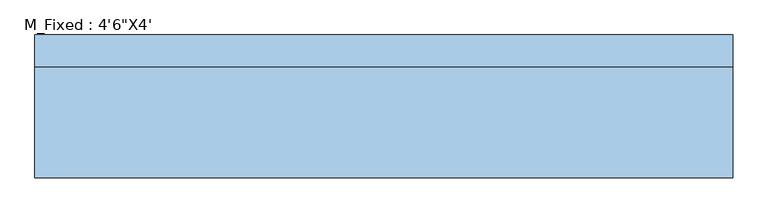
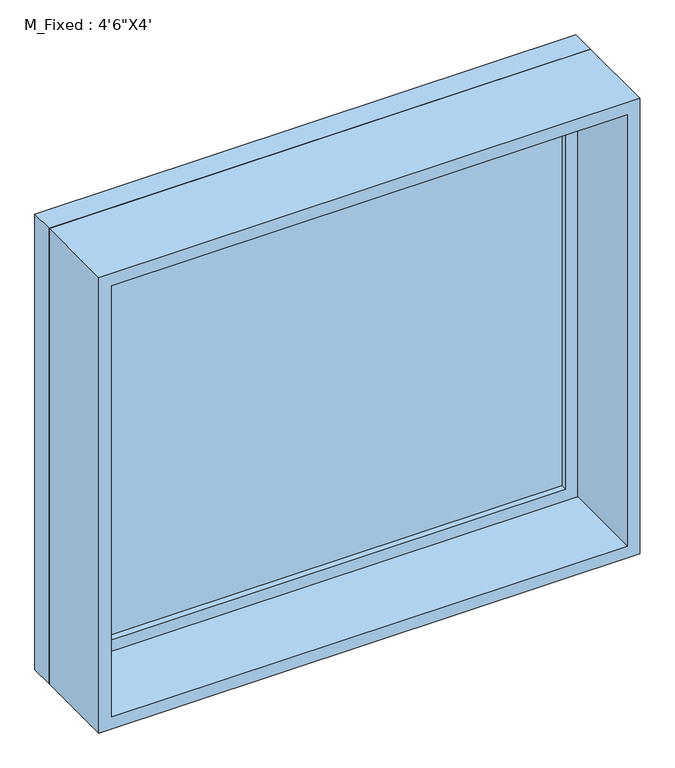
"""IFC4 building model written with IfcOpenShell, lengths in millimetres: window geometry."""

from ifc_helpers import new_model, si_unit, frame, origin, place, context, project, spatial, polyline, outline, extrude, source, transform, mapped, element, save


def window_6cb3df29(model_context):
    return source(origin(), model_context, "Body", "SweptSolid", [
        extrude(outline(polyline([(-622.8, 118.4), (622.8, 118.4), (622.8, 106.4), (-622.8, 106.4), (-622.8, 118.4)])), frame((0.0, 0.0, 977.4), z_axis=(0.0, 0.0, 1.0), x_axis=(1.0, 0.0, 0.0)), (0.0, 0.0, 1.0), 1093.2),
        extrude(outline(polyline([(2114.6, -666.8), (933.4, -666.8), (933.4, 666.8), (2114.6, 666.8), (2114.6, -666.8)]), holes=[polyline([(2070.6, -622.8), (2070.6, 622.8), (977.4, 622.8), (977.4, -622.8), (2070.6, -622.8)])]), frame((0.0, 90.4, 0.0), z_axis=(0.0, 1.0, 0.0), x_axis=(0.0, 0.0, 1.0)), (0.0, 0.0, 1.0), 44.0),
        extrude(outline(polyline([(2133.6, -685.8), (914.4, -685.8), (914.4, 685.8), (2133.6, 685.8), (2133.6, -685.8)]), holes=[polyline([(2114.6, -666.8), (2114.6, 666.8), (933.4, 666.8), (933.4, -666.8), (2114.6, -666.8)])]), frame((0.0, 90.4, 0.0), z_axis=(0.0, 1.0, 0.0), x_axis=(0.0, 0.0, 1.0)), (0.0, 0.0, 1.0), 63.0),
        extrude(outline(polyline([(2133.6, -685.8), (914.4, -685.8), (914.4, 685.8), (2133.6, 685.8), (2133.6, -685.8)]), holes=[polyline([(2101.6, -653.8), (2101.6, 653.8), (946.4, 653.8), (946.4, -653.8), (2101.6, -653.8)])]), frame((0.0, -127.4, 0.0), z_axis=(0.0, 1.0, 0.0), x_axis=(0.0, 0.0, 1.0)), (0.0, 0.0, 1.0), 217.8),
    ])


if __name__ == "__main__":
    model = new_model("IFC4")
    model_context = context("Model", 3, world=origin())
    ifc_project = project(units=[si_unit("LENGTHUNIT", "METRE", prefix="MILLI")], contexts=[model_context])
    site = spatial("IfcSite", under=ifc_project)
    building = spatial("IfcBuilding", under=site)
    placement = place(None, origin())
    window_shape = window_6cb3df29(model_context)
    element("IfcWindow", 1, ObjectType="M_Fixed : 4'6\"X4'", at=placement, inside=building, context=model_context, shape_type="MappedRepresentation", body=[
        mapped(window_shape, transform((0.0, 0.0, 0.0), x_axis=(1.0, 0.0, 0.0), y_axis=(0.0, 1.0, 0.0), z_axis=(0.0, 0.0, 1.0))),
    ])
    save(model, "model.ifc")

# Revit data of these elements
# Type "M_Fixed : 4'6\"X4'"
#   Construction Type Id = "DG-DR"
#   Analytic Construction = "Double glazing - domestic"
#   Type Mark = "19"
#   Visual Light Transmittance = 0.81
#   Solar Heat Gain Coefficient = 0.76
#   Heat Transfer Coefficient (U) = 3.1292 W/(m²·K)
#   Height = 4' - 0"
#   Default Sill Height = 3' - 0"
#   Width = 4' - 6"
#   Window Inset = 0' - 0.74803"
#   Wall Closure = 2
#   Frame Exterior Material = Sash
#   Frame Interior Material = Sash
#   Glass Pane Material = Glass
#   Sash = Sash
# Element 1 (IfcWindow, "M_Fixed : 4'6\"X4'")
#   Materials on its faces: "Sash", "Glass"
# Materials
#   "Sash": class "Wood", colour RGB 136 99 55, transparency 0
#   "Glass": class "Glass", colour RGB 218 227 224, transparency 0.85, Description = "Soda Lime Glass", Cost = 0
